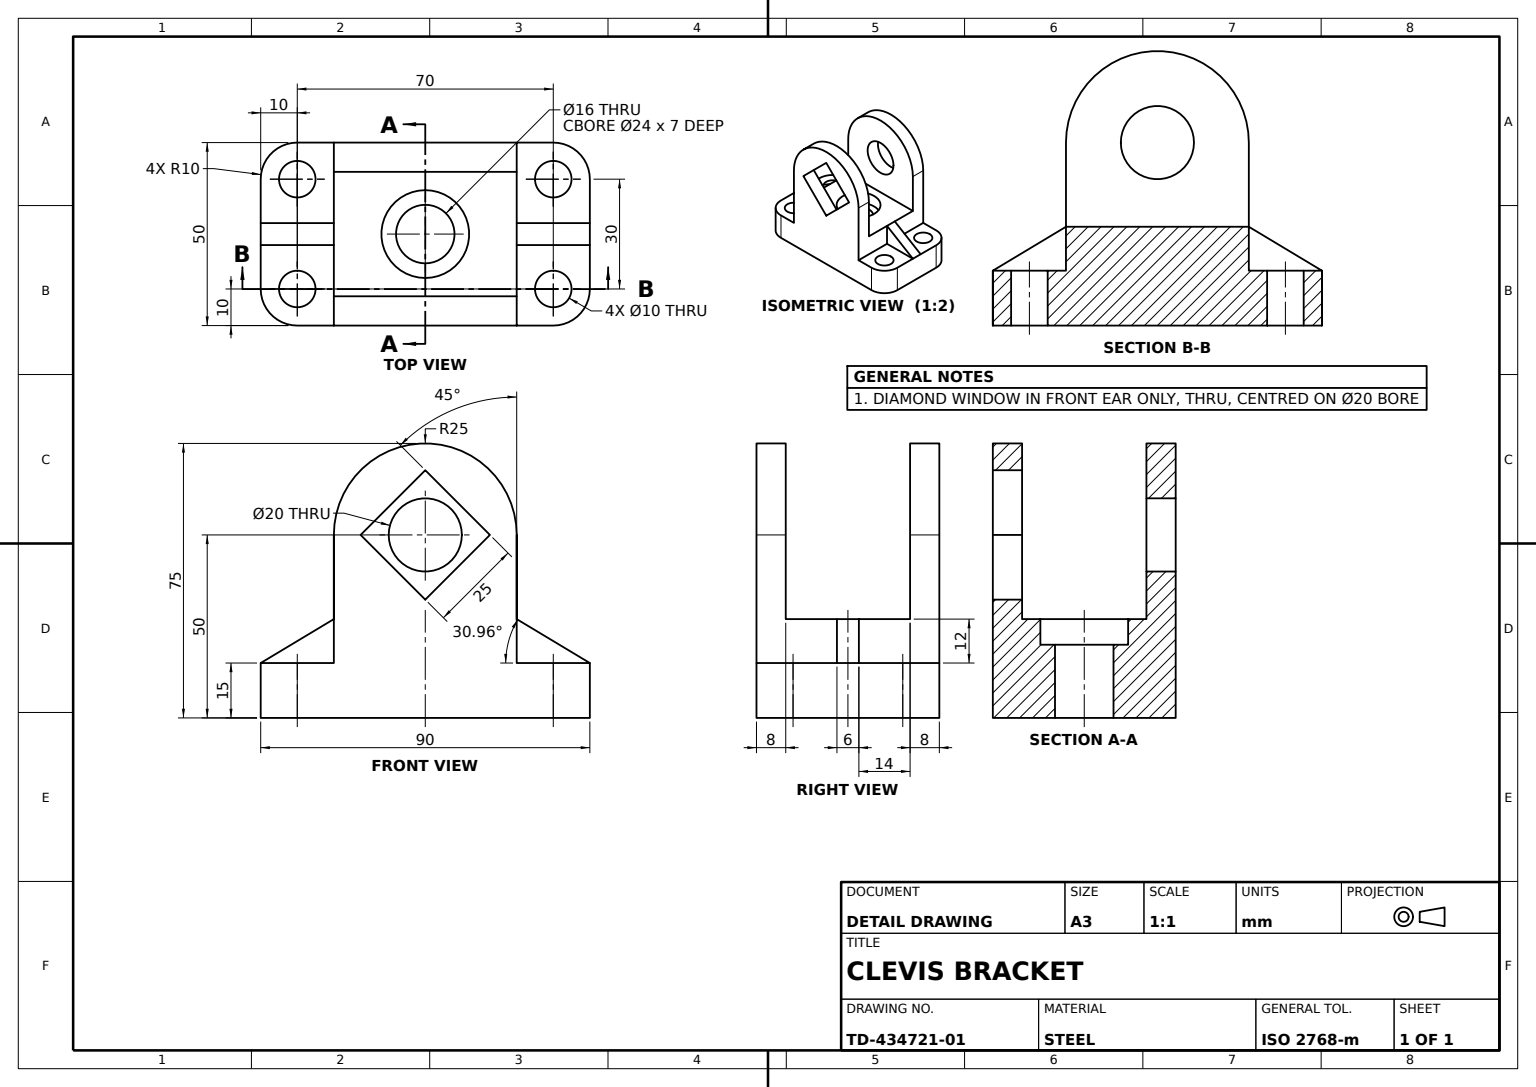
from build123d import *

# Parameters (mm, degrees)
BASE_PLATE_SKETCH_R              = 5
BASE_PLATE_DEPTH                 = 15
CLEVIS_EAR_DEPTH                 = 8
CENTRE_CUT_DEPTH                 = 8
PIN_BORE_SKETCH_R                = 10
PIN_BORE_20_DEPTH                = 8
EAR_BOSS_SKETCH_W                = 50
EAR_BOSS_SKETCH_H                = 34
EAR_BOSS_DEPTH                   = 12
GUSSET_RIB_REACH                 = 92.967
GUSSET_SKETCH_WALL_W             = 207.257861566
GUSSET_SKETCH_WALL_H             = 6
COUNTERBORED_HOLE_16_D           = 16
COUNTERBORED_HOLE_16_DEPTH       = 49.839743178
COUNTERBORED_HOLE_16_CBORE_D     = 24
COUNTERBORED_HOLE_16_CBORE_DEPTH = 7


with BuildPart() as part:
    # Base Plate Sketch → Base Plate (new body)
    with BuildSketch(Plane(origin=(0, 0, 0), x_dir=(1, 0, 0), z_dir=(0, 1, 0))):
        with BuildLine():
            Line((-35, -25), (35, -25))
            ThreePointArc((35, -25), (42.071067812, -22.071067812), (45, -15))
            Line((45, -15), (45, 15))
            ThreePointArc((45, 15), (42.071067812, 22.071067812), (35, 25))
            Line((35, 25), (-35, 25))
            ThreePointArc((-35, 25), (-42.071067812, 22.071067812), (-45, 15))
            Line((-45, 15), (-45, -15))
            ThreePointArc((-45, -15), (-42.071067812, -22.071067812), (-35, -25))
        make_face()
        with Locations(Location((-35, 15, 0), (0, 0, 270))):
            Circle(BASE_PLATE_SKETCH_R, mode=Mode.SUBTRACT)
        with Locations(Location((35, 15, 0), (0, 0, 270))):
            Circle(BASE_PLATE_SKETCH_R, mode=Mode.SUBTRACT)
        with Locations(Location((-35, -15, 0), (0, 0, 270))):
            Circle(BASE_PLATE_SKETCH_R, mode=Mode.SUBTRACT)
        with Locations(Location((35, -15, 0), (0, 0, 270))):
            Circle(BASE_PLATE_SKETCH_R, mode=Mode.SUBTRACT)
    extrude(amount=BASE_PLATE_DEPTH)

    # Clevis Ear Sketch → Clevis Ear (add)
    with BuildSketch(Plane.XY.offset(25)):
        with BuildLine():
            Line((-25, 15), (-25, 50))
            ThreePointArc((-25, 50), (0, 75), (25, 50))
            Line((25, 50), (25, 15))
            Line((25, 15), (-25, 15))
        make_face()
    clevis_ear = extrude(amount=-CLEVIS_EAR_DEPTH)

    # Clevis Ear Mirror: Clevis Ear across plane
    add(clevis_ear.mirror(Plane.XY))

    # Centre Cut Sketch → Centre Cut (cut)
    with BuildSketch(Plane.XY.offset(25)):
        Polygon((-17.67766953, 50), (0, 67.67766953), (17.67766953, 50), (0, 32.32233047), align=None)
    extrude(amount=-CENTRE_CUT_DEPTH, mode=Mode.SUBTRACT)

    # Pin Bore Sketch → Pin Bore Ø20 (cut)
    with BuildSketch(Plane(origin=(0, 0, -25), x_dir=(-1, 0, 0), z_dir=(0, 0, -1))):
        with Locations((0, 50)):
            Circle(PIN_BORE_SKETCH_R)
    extrude(amount=-PIN_BORE_20_DEPTH, mode=Mode.SUBTRACT)

    # Ear Boss Sketch → Ear Boss (add)
    with BuildSketch(Plane(origin=(0, 15, 0), x_dir=(1, 0, 0), z_dir=(0, 1, 0))):
        Rectangle(EAR_BOSS_SKETCH_W, EAR_BOSS_SKETCH_H)
    extrude(amount=EAR_BOSS_DEPTH)

    # Gusset Sketch wall → Gusset Rib (add, up to next)
    with BuildSketch(Plane(origin=(35, 21, 0), x_dir=(0.857492925713, -0.514495755428, 0), z_dir=(0.514495755428, 0.857492925713, 0)), mode=Mode.PRIVATE) as gusset_rib_sk1:
        Rectangle(GUSSET_SKETCH_WALL_W, GUSSET_SKETCH_WALL_H)
    gusset_rib_tool1 = extrude(gusset_rib_sk1.sketch, amount=-GUSSET_RIB_REACH, mode=Mode.PRIVATE) - part.part
    gusset_rib = gusset_rib_tool1.solids().sort_by_distance((35, 21, 0))[0]
    add(gusset_rib)

    # Gusset Rib Mirror: Gusset Rib across plane
    add(gusset_rib.mirror(Plane(origin=(0, 0, 0), x_dir=(0, 0, 1), z_dir=(1, 0, 0))))

    # Counterbored Hole Ø16
    with Locations(Plane.ZX.offset(27)):
        with Locations((0, 0)):
            CounterBoreHole(COUNTERBORED_HOLE_16_D / 2, COUNTERBORED_HOLE_16_CBORE_D / 2, COUNTERBORED_HOLE_16_CBORE_DEPTH, depth=COUNTERBORED_HOLE_16_DEPTH)


solid = part.part
